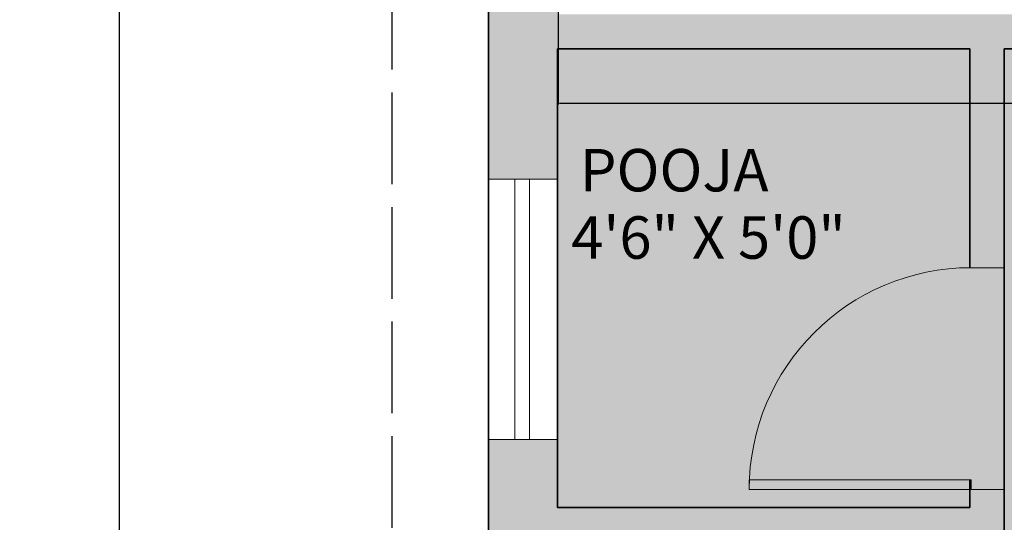
# Model space of a CAD drawing. Units: inches. Extents: x 1316 to 1777, y 813 to 1650.
# Tile 6 of 22: x 1316 to 1445, y 1368 to 1434. Entities that reach past the tile are written whole.
import ezdxf

# ---------------------------------------------------------------- set-up
doc = ezdxf.new("R2010")
doc.units = ezdxf.units.IN
doc.header["$MEASUREMENT"] = 0
doc.linetypes.add('ACAD_ISO02W100', pattern=[15, 12, -3])
for name, color, linetype, lineweight in [('A-ANNO-DIMS', 2, 'Continuous', 18), ('A-AREA-IDEN', 7, 'Continuous', 18), ('A-DOOR', 4, 'Continuous', 18), ('A-DOOR-PATT', 253, 'Continuous', 13), ('A-WALL-PATT', 250, 'Continuous', 13), ('C-PROP', 8, 'ACAD_ISO02W100', 25), ('walls', 250, 'Continuous', 35), ('windows', 141, 'Continuous', 18)]:
    doc.layers.add(name, color=color, linetype=linetype, lineweight=lineweight)
doc.layers.add('A-FLOR-PATT', color=254, linetype='Continuous', lineweight=13, true_color=0xfeeab9)
doc.styles.get("Standard").update_dxf_attribs({"font": 'arial.ttf'})
doc.dimstyles.get("Standard").update_dxf_attribs({"dimtxt": 7, "dimasz": 0.18, "dimexe": 0.18, "dimexo": 0.0625, "dimgap": 0.09, "dimtad": 0, "dimtih": 1, "dimtoh": 1, "dimzin": 0, "dimdsep": 46, "dimlunit": 3, "dimtxsty": 'Standard', "dimcen": 0.09, "dimadec": 0, "dimazin": 0, "dimtfac": 1, "dimtofl": 0, "dimtmove": 0, "dimatfit": 3, "dimfxl": 1, "dimtolj": 1, "dimtzin": 0, "dimarcsym": 0})

# ---------------------------------------------------------------- blocks, each defined once
blk = doc.blocks.new('*U15')
for p, q in [((0, 0), (-1e-16, -5.999999999999999)), ((40, -6e-16), (40, -6))]:
    blk.add_line(p, q)
blk.add_lwpolyline([(0, 0), (5.6e-15, 40), (1.750000000000007, 40), (1.749999999999998, -7e-16)], close=True)
blk.add_arc((0, 0), 40, 0, 90)
blk = doc.blocks.new('*D23')
at = {"layer": 'A-ANNO-DIMS', "color": 0, "lineweight": -2, "transparency": 16777216}
for p, q in [((1328.466746604303, 1604.172951843256), (1328.865516882555, 1604.172951843256)), ((1328.685516882555, 1603.992951843256), (1328.685516882555, 1282.594977494184)), ((1328.685516882555, 953.868981317008), (1328.685516882555, 1275.26695566608)), ((1328.466746604303, 953.688981317008), (1328.865516882556, 953.688981317008))]:
    blk.add_line(p, q, dxfattribs=at)
at = {"layer": 'A-ANNO-DIMS', "color": 0, "transparency": 16777216}
for points in [[(1328.655516882555, 1603.992951843256), (1328.715516882555, 1603.992951843256), (1328.685516882555, 1604.172951843256)], [(1328.655516882556, 953.868981317008), (1328.715516882555, 953.868981317008), (1328.685516882555, 953.688981317008)]]:
    blk.add_solid(points, dxfattribs=at)
at = {"layer": 'Defpoints', "color": 0, "transparency": 16777216}
for p in [(1328.404246604303, 1604.172951843256), (1328.404246604303, 953.688981317008), (1328.685516882555, 953.688981317008)]:
    blk.add_point(p, dxfattribs=at)
at = {"layer": 'A-ANNO-DIMS', "color": 0, "transparency": 16777216, "insert": (1328.685516882555, 1278.930966580132), "char_height": 7, "width": 24.3281036834925, "attachment_point": 5}
blk.add_mtext('\\A1;47\'-0"', dxfattribs=at)
blk = doc.blocks.new('*D30')
at = {"layer": 'A-ANNO-DIMS', "color": 0, "lineweight": -2, "transparency": 16777216}
for p, q in [((1386.153353095512, 1434.699095169867), (1386.153353095512, 1422.57802783725)), ((1466.177135312958, 1434.699095169867), (1466.177135312958, 1422.57802783725)), ((1386.333353095512, 1422.75802783725), (1465.997135312959, 1422.75802783725)), ((1466.177135312958, 1422.75802783725), (1466.357135312958, 1422.75802783725))]:
    blk.add_line(p, q, dxfattribs=at)
at = {"layer": 'A-ANNO-DIMS', "color": 0, "transparency": 16777216}
for points in [[(1386.333353095512, 1422.78802783725), (1386.333353095512, 1422.72802783725), (1386.153353095512, 1422.75802783725)], [(1465.997135312959, 1422.78802783725), (1465.997135312959, 1422.72802783725), (1466.177135312958, 1422.75802783725)]]:
    blk.add_solid(points, dxfattribs=at)
at = {"layer": 'Defpoints', "color": 0, "transparency": 16777216}
for p in [(1386.153353095512, 1434.761595169867), (1466.177135312958, 1434.761595169867), (1466.177135312958, 1422.75802783725)]:
    blk.add_point(p, dxfattribs=at)
at = {"layer": 'A-ANNO-DIMS', "color": 0, "transparency": 16777216, "insert": (1518.078103935059, 1422.75802783725), "char_height": 7, "attachment_point": 5}
blk.add_mtext('\\A1;WARDROBE 6\'-8" TYP.', dxfattribs=at)
blk = doc.blocks.new('*D36')
at = {"layer": 'A-ANNO-DIMS', "color": 0, "lineweight": -2, "transparency": 16777216}
for p, q in [((1416.108011424953, 1349.392697936214), (1416.108011424953, 1345.951925450247)), ((1438.2631613314, 1349.392697936214), (1438.2631613314, 1345.951925450247)), ((1416.288011424953, 1346.131925450247), (1438.0831613314, 1346.131925450247)), ((1438.2631613314, 1346.131925450247), (1438.443161331401, 1346.131925450247))]:
    blk.add_line(p, q, dxfattribs=at)
at = {"layer": 'A-ANNO-DIMS', "color": 0, "transparency": 16777216}
for points in [[(1416.288011424953, 1346.161925450247), (1416.288011424953, 1346.101925450247), (1416.108011424953, 1346.131925450247)], [(1438.0831613314, 1346.161925450247), (1438.0831613314, 1346.101925450247), (1438.2631613314, 1346.131925450247)]]:
    blk.add_solid(points, dxfattribs=at)
at = {"layer": 'Defpoints', "color": 0, "transparency": 16777216}
for p in [(1416.108011424953, 1349.455197936214), (1438.2631613314, 1349.455197936214), (1438.2631613314, 1346.131925450247)]:
    blk.add_point(p, dxfattribs=at)
at = {"layer": 'A-ANNO-DIMS', "color": 0, "transparency": 16777216, "insert": (1493.434934864825, 1346.131925450247), "char_height": 7, "attachment_point": 5}
blk.add_mtext('\\A1;WALL BASIN 1\'-10" TYP.', dxfattribs=at)

msp = doc.modelspace()

# ---------------------------------------------------------------- hatches: boundary and pattern name
at = {"layer": 'A-DOOR-PATT'}
h = msp.add_hatch(color=256, dxfattribs=at)
h.dxf.hatch_style = 1
h.paths.add_polyline_path([(1440.064450217018, 1373.459281729462), (1411.195884528974, 1373.459281729462, 0.0109414287710455), (1411.168078720428, 1372.18876759644), (1440.064450217018, 1372.18876759644)])
h.paths.add_polyline_path([(1505.845136951899, 1441.821674157348), (1476.976571263855, 1441.821674157348, 0.0109414287710455), (1476.948765455309, 1440.551160024325), (1505.845136951899, 1440.551160024325)])
h.paths.add_polyline_path([(1510.345136951899, 1469.591483064839), (1505.989088495822, 1469.591483064839, 0.0012392441961977), (1505.845136951899, 1469.59112628206), (1505.845136951899, 1441.821674157348), (1505.989088495822, 1441.821674157348), (1505.989088495822, 1440.551160024325), (1510.345136951899, 1440.551160024325)])
at = {"layer": 'A-FLOR-PATT'}
h = msp.add_hatch(color=256, dxfattribs=at)
h.dxf.hatch_style = 1
h.paths.add_polyline_path([(1567.673142217696, 1281.369300926962), (1651.673142217696, 1281.369300926962), (1651.673142217696, 1365.369300926962), (1597.673142217696, 1365.369300926962), (1597.673142217696, 1429.869300926962), (1570.345136951899, 1429.869300926962), (1570.345136951899, 1471.869300926962), (1510.345136951899, 1471.869300926962), (1510.345136951899, 1429.869300926962), (1444.564450217018, 1429.869300926962), (1444.564450217018, 1322.882360660317), (1444.564450217018, 1300.087519887597), (1510.564450217018, 1300.087519887597), (1510.564450217018, 1295.093869264817), (1510.564450217018, 1240.869300926962), (1386.064450217018, 1240.869300926962), (1386.064450217018, 1171.184826128129), (1400.961298831769, 1171.184826128129), (1400.961298831769, 1106.74181853581), (1386.064450217018, 1106.74181853581), (1386.064450217018, 1072.869300926962), (1510.564450217018, 1072.869300926962), (1510.564450217018, 1040.172951843256), (1541.068383692007, 1040.172951843256, -0.367085007058701), (1572.764174999282, 1069.546549507821), (1572.764174999282, 1069.578525976929), (1574.225256623933, 1069.578525976929), (1574.225256623933, 1040.172951843256), (1616.037285953149, 1040.172951843256), (1616.037285953149, 1086.627161740109), (1616.037285953149, 1103.704513499145), (1613.066060418845, 1105.234780569291), (1616.037285953149, 1106.685539866415), (1616.037285953149, 1123.869300926962), (1567.673142217696, 1123.869300926962)])
h.paths.add_polyline_path([(1508.987494855724, 1198.018101264616), (1511.117481528599, 1198.018101264616), (1511.117481528599, 1200.148087937491), (1532.594847146751, 1200.148087937491), (1532.594847146751, 1198.018101264616), (1534.724833819626, 1198.018101264616), (1534.724833819626, 1176.008238978245), (1530.464860473877, 1176.008238978245), (1530.464860473877, 1176.71823453587), (1513.247468201473, 1176.71823453587), (1513.247468201473, 1176.008238978245), (1508.987494855724, 1176.008238978245)], flags=16)
h.paths.add_polyline_path([(1505.978911344017, 1151.314990471522), (1521.503967005494, 1151.314990471522), (1521.503967005494, 1123.622553675171), (1505.978911344017, 1123.622553675171)], flags=16)
h.paths.add_polyline_path([(1507.734238645614, 1150.100746953806, -1), (1506.932299902515, 1150.100746953806, -1)], flags=0)
h.paths.add_polyline_path([(1512.288074001727, 1138.353334368216), (1512.279600715468, 1138.392440283947), (1512.219350358134, 1138.376242249414)], flags=0)
h.paths.add_polyline_path([(1511.538708600003, 1138.926307509397), (1511.801586230713, 1138.967144364025), (1511.816822451641, 1139.269704188439), (1511.606794574277, 1139.246286533845)], flags=0)
h.paths.add_polyline_path([(1513.744555260512, 1140.234298321423), (1513.680232363733, 1139.885116881769), (1514.013725426534, 1140.045442118172), (1513.85452204526, 1140.307851476896)], flags=0)
h.paths.add_polyline_path([(1513.759454991183, 1139.088508933479), (1514.004707571892, 1139.255238426424), (1513.806733823314, 1139.482778214552), (1513.564128907831, 1139.327271464974)], flags=0)
h.paths.add_polyline_path([(1514.219475210051, 1138.385213274156), (1514.335730050378, 1138.330012877603), (1514.544443105969, 1138.319719602207), (1514.802071501717, 1138.873746829037), (1514.451386945615, 1138.715560522777)], flags=0)
h.paths.add_polyline_path([(1514.576784523415, 1137.439218133731), (1514.572807725035, 1137.400121795131), (1514.699202201671, 1137.400121795131), (1514.696265725507, 1137.401958254237)], flags=0)
h.paths.add_polyline_path([(1512.259630054145, 1136.199252443718), (1512.198645006043, 1136.399020086717), (1512.031969302785, 1136.324884611944), (1512.095408670439, 1136.101205019573), (1512.257489338984, 1136.192116726515)], flags=0)
h.paths.add_polyline_path([(1512.643663084783, 1137.273739653883), (1512.355504649132, 1137.230281342332), (1512.431954114942, 1137.048783229095), (1512.702875297586, 1137.092989450977)], flags=0)
h.paths.add_polyline_path([(1513.048588650928, 1137.592520798729), (1512.979298324136, 1137.799799709794), (1512.842806872769, 1137.757466697763), (1512.887278702865, 1137.556025839099)], flags=0)
h.paths.add_polyline_path([(1513.269281623239, 1138.555876366321), (1513.570749546786, 1137.962332598873), (1513.458764523686, 1136.814048268166), (1513.212081965274, 1137.877990637943), (1513.032322366809, 1138.442602014432)], flags=0)
h.paths.add_polyline_path([(1514.891020715756, 1136.377090047208), (1514.695899864911, 1136.400535518201), (1514.682939550409, 1136.245500587688), (1514.870369662043, 1136.165423867704)], flags=0)
h.paths.add_polyline_path([(1514.142311807212, 1137.292647657223), (1514.047049214511, 1136.74320071616), (1514.270411313405, 1136.750949401328), (1514.327746372416, 1137.265481105849)], flags=0)
h.paths.add_polyline_path([(1515.361925908058, 1138.975942407129), (1515.333738674027, 1138.638448296537), (1515.595602136156, 1138.588081597507), (1515.627104749056, 1138.931608018565)], flags=0)
h.paths.add_polyline_path([(1537.284795120854, 1177.912388692567), (1537.994790678479, 1177.912388692567), (1537.994790678479, 1195.129780964971), (1537.284795120854, 1195.129780964971), (1537.284795120854, 1199.38975431072), (1559.294657407225, 1199.38975431072), (1559.294657407225, 1197.259767637845), (1561.4246440801, 1197.259767637845), (1561.4246440801, 1175.782402019693), (1559.294657407225, 1175.782402019693), (1559.294657407225, 1173.652415346818), (1559.378615070445, 1173.652415346818), (1559.378615070445, 1171.514303738793), (1561.51672667847, 1171.514303738793), (1561.51672667847, 1098.818509065945), (1559.378615070445, 1098.818509065945), (1559.378615070445, 1096.68039745792), (1537.284795120854, 1096.68039745792), (1537.284795120854, 1100.95662067397), (1537.997498990196, 1100.95662067397), (1537.997498990196, 1169.376192130768), (1537.284795120854, 1169.376192130768), (1537.284795120854, 1173.652415346818)], flags=16)
h.paths.add_polyline_path([(1518.623279367581, 1345.565265318288), (1519.133216999197, 1345.479657117201), (1519.133247129367, 1345.484585273925), (1518.623292796693, 1345.567461813277)], flags=16)
h.paths.add_polyline_path([(1518.798043157878, 1374.150014517315), (1519.307980789494, 1374.064406316228), (1519.308010919664, 1374.069334472953), (1518.79805658699, 1374.152211012305)], flags=16)
h.paths.add_polyline_path([(1537.763945546351, 1413.501272593833), (1537.678419015976, 1412.991334462891), (1537.683273643974, 1412.991304782267), (1537.76615767817, 1413.501259069119)], flags=16)
h.paths.add_polyline_path([(1572.904903294898, 1373.821409718101), (1573.926762419731, 1373.974678074354), (1574.026627442758, 1390.308820473798), (1573.007147246318, 1390.474521481455), (1573.006718884663, 1390.474591095266)], flags=16)
h.paths.add_polyline_path([(1572.730139504601, 1345.236660519073), (1573.751998629434, 1345.389928875326), (1573.851863652461, 1361.72407127477), (1572.832383456021, 1361.889772282427), (1572.831955094366, 1361.889841896238)], flags=16)
h.paths.add_polyline_path([(1537.210658487583, 1322.64259197221), (1537.363943428096, 1321.620732745983), (1553.69808582754, 1321.520867722956), (1553.863838585734, 1322.540776390265)], flags=16)
h.paths.add_polyline_path([(1535.907853535946, 1331.328394679552), (1527.214399285865, 1331.381545435045), (1527.663791889487, 1404.885186232545), (1564.415612288236, 1404.660489930734), (1563.966219684615, 1331.156849133235), (1555.272745017813, 1331.210000013553), (1553.946716560728, 1323.050730714162), (1537.134020158137, 1323.153521560007)], flags=16)
h.paths.add_polyline_path([(1536.149948378398, 1336.502989385165), (1536.235164066325, 1337.571577967879), (1536.323287084786, 1338.628101895201), (1536.410786509507, 1339.662781903015), (1536.494625364907, 1340.6698173033), (1536.573878305868, 1341.65983134291), (1536.648126641431, 1342.647834135966), (1536.716972722469, 1343.648937760143), (1536.780017027388, 1344.677948027938), (1536.836830656389, 1345.749875115879), (1536.91349345135, 1347.47536960008), (1536.930181129876, 1348.082213381731), (1536.86671979596, 1346.313806322279), (1536.754065794645, 1344.188314997416), (1536.618602559507, 1342.21851898877), (1536.494625364906, 1340.669817303289), (1536.410786509508, 1339.662781903024), (1536.323287084785, 1338.628101895196), (1536.235164066325, 1337.571577967878), (1536.149948378398, 1336.502989385167), (1536.071202820108, 1335.432319400725), (1536.002480605875, 1334.369653419014), (1535.917201218224, 1332.754159960459), (1535.909282823342, 1332.307756473361), (1535.96435308899, 1333.780079645636), (1536.071202820108, 1335.432319400726)], flags=0)
h.paths.add_polyline_path([(1540.411728678358, 1338.345220732376), (1540.538507986221, 1339.036732867615), (1540.667450686668, 1339.758144792479), (1540.798139602249, 1340.51803480286), (1540.930104638842, 1341.324675241543), (1541.06290820131, 1342.186644529235), (1541.195663950278, 1343.109256879628), (1541.325751198274, 1344.084667215432), (1541.450112594895, 1345.102072455087), (1541.565699126105, 1346.150363189455), (1541.669432399664, 1347.218634373414), (1541.758274858692, 1348.295980712192), (1541.829158319786, 1349.371497098253), (1541.87902418423, 1350.434176273261), (1541.905658245644, 1351.475864398132), (1541.910264078201, 1352.499718972741), (1541.894848813054, 1353.511751165878), (1541.861450207875, 1354.517971959091), (1541.812104772023, 1355.524188157142), (1541.748831093802, 1356.536615043187), (1541.673675267255, 1357.560957271187), (1541.551221046702, 1359.062282646612), (1541.495486505545, 1359.670454934914), (1541.588655256529, 1358.603328035907), (1541.721318618915, 1356.976835527602), (1541.846114060333, 1354.980013725856), (1541.912433480836, 1352.981966815021), (1541.903299375855, 1350.951498912638), (1541.805645357175, 1348.870418133965), (1541.627733180341, 1346.712969607265), (1541.39605931794, 1344.611846225434), (1541.135168242209, 1342.655652549989), (1540.871929016276, 1340.947082961546), (1540.617179283622, 1339.465841984599), (1540.411728678363, 1338.345220732389), (1540.287580984743, 1337.67502977883), (1540.166494164132, 1337.01788791383), (1540.048925605183, 1336.365114503449), (1539.936674201221, 1335.710368832696), (1539.836864251217, 1335.055036635329), (1539.758020939376, 1334.402536924379), (1539.708629238703, 1333.756391050932), (1539.697173498044, 1333.120018277682), (1539.75093556766, 1332.162191347439), (1539.822087714565, 1331.89006440645), (1539.690956844971, 1332.774679737417), (1539.713650637448, 1334.035332547662), (1539.86680860596, 1335.30285325234), (1540.085210789094, 1336.576760560778), (1540.287580984743, 1337.67502977883)], flags=0)
h.paths.add_polyline_path([(1545.598581542273, 1331.583674047033), (1545.601408931398, 1331.616855477121), (1545.614142276281, 1331.689058908809), (1545.736718477884, 1332.197227143153), (1545.766951209007, 1332.331509735297), (1545.840044120643, 1332.681341212682), (1545.924609388668, 1333.114205605127), (1546.015565858785, 1333.613901317454), (1546.107830504227, 1334.163920489319), (1546.196310713542, 1334.747857411176), (1546.27592408412, 1335.349306311069), (1546.341588213349, 1335.951861417042), (1546.388220074462, 1336.539014868746), (1546.411904372759, 1337.098233262493), (1546.413511757999, 1337.631655211558), (1546.395048737181, 1338.145189796344), (1546.358553067975, 1338.644847998394), (1546.30606313221, 1339.136742887642), (1546.239595021565, 1339.626681393686), (1546.161196702551, 1340.120674435653), (1546.072884891005, 1340.624631031533), (1545.887738197254, 1341.63015699768), (1545.717659533451, 1342.62070013092), (1545.546853733249, 1343.94500888803), (1545.431881256549, 1345.533720124316), (1545.403899849759, 1347.401905451854), (1545.417510423816, 1348.013069267128), (1545.410556413592, 1346.957478372932), (1545.425070640934, 1345.988432507364), (1545.462877367243, 1345.105410056077), (1545.521092971858, 1344.300975918152), (1545.595702123642, 1343.566272620922), (1545.68263719895, 1342.892238827028), (1545.777872657803, 1342.270017126221), (1545.877351709551, 1341.690648207114), (1545.977037981224, 1341.145172633476), (1546.133225269608, 1340.296924301995), (1546.32712189736, 1339.07516870602), (1546.43378476773, 1337.614859053002), (1546.377188266119, 1336.278538916938), (1546.246417261819, 1335.078542247844), (1546.032296532176, 1333.665423983985), (1545.840044120643, 1332.681341212682), (1545.766951209007, 1332.331509735297)], flags=0)
h.paths.add_polyline_path([(1551.802739251137, 1337.655775652498), (1551.96257269545, 1338.249893918501), (1552.102195298518, 1338.801154932478), (1552.224958021371, 1339.338328209144), (1552.330696453755, 1339.864579612065), (1552.418402861907, 1340.377056720641), (1552.487067639598, 1340.872600849098), (1552.535672844225, 1341.34835963925), (1552.563199284875, 1341.801276556129), (1552.568639227787, 1342.228499179132), (1552.550972857889, 1342.626868884903), (1552.509678498417, 1342.994551203202), (1552.446288501197, 1343.33337442512), (1552.362792521005, 1343.646491244529), (1552.261208966661, 1343.936747902882), (1552.143557495304, 1344.207194818415), (1552.011836098078, 1344.460678357413), (1551.868075265113, 1344.700350964085), (1551.746105860759, 1344.881722683215), (1550.887297650741, 1346.05192221882), (1550.42788872704, 1347.125680184261), (1550.183287427721, 1348.353333686171), (1550.047936052465, 1349.632359022536), (1549.978096005541, 1351.223542107026), (1549.974102148838, 1353.140827975589), (1549.989226669163, 1353.748427546368), (1549.975058438592, 1352.681752708607), (1549.977087298692, 1351.70778065901), (1549.995607655661, 1350.824569845699), (1550.030618304039, 1350.026913573531), (1550.082058657804, 1349.309911787039), (1550.149928759809, 1348.668561967865), (1550.234168024029, 1348.097964060535), (1550.334775869163, 1347.593013458303), (1550.451691709185, 1347.148810105696), (1550.584412233058, 1346.759844100773), (1550.73038050297, 1346.418678345312), (1550.88655602074, 1346.117266144286), (1551.049909745336, 1345.847764917032), (1551.217401178577, 1345.602127968521), (1551.385990446439, 1345.372410692116), (1551.55262809021, 1345.150770631988), (1552.000038284146, 1344.537104232464), (1552.453505275841, 1343.494713960715), (1552.591463897673, 1342.266339273388), (1552.508711326437, 1340.904737898757), (1552.245597777252, 1339.367339734202), (1551.924893638995, 1338.101128644033), (1551.618511514029, 1336.984114361546), (1551.405674157756, 1336.200020283199), (1551.009764092749, 1334.698598399404), (1550.877399289293, 1334.154667887629), (1551.263664389663, 1335.676855458292), (1551.618511514027, 1336.984114361536)], flags=0)
h.paths.add_polyline_path([(1558.642358998526, 1348.348341932098), (1558.795153425402, 1348.811416841303), (1558.918173552255, 1349.215358215379), (1559.008026171039, 1349.574581801048), (1559.061298904339, 1349.903707646641), (1559.075825921932, 1350.214183320864), (1559.054343192669, 1350.505992096326), (1559.00083323259, 1350.775944766007), (1558.919250427844, 1351.021260663692), (1558.81356708563, 1351.238750644777), (1558.687756761463, 1351.425429741436), (1558.545793010855, 1351.578312985846), (1558.391628971643, 1351.694415535011), (1558.228764001313, 1351.771674150153), (1558.05869086465, 1351.812121548804), (1557.882428128411, 1351.81871217754), (1557.700994359352, 1351.79440048294), (1557.515397915392, 1351.742140973996), (1557.326668820441, 1351.665092211649), (1557.135793766425, 1351.566004652943), (1556.943823194933, 1351.44803673399), (1556.751584825563, 1351.314654529213), (1556.741969848742, 1351.307485185875), (1556.174649390243, 1350.878470713214), (1555.982386678774, 1350.741107061228), (1555.790208852573, 1350.61762743028), (1555.103431920574, 1350.247624890473), (1554.019478994433, 1350.696346369238), (1553.658410413117, 1351.73359972735), (1553.592207666961, 1352.861368347784), (1553.704659497418, 1354.248209262139), (1553.753119918252, 1354.656598557367), (1553.684819216316, 1354.00352392911), (1553.637913725648, 1353.425049987856), (1553.614699631385, 1352.917691559993), (1553.614827379228, 1352.476039895736), (1553.637249468889, 1352.094077959223), (1553.680938817757, 1351.765788589762), (1553.744858758541, 1351.485256777466), (1553.82798220863, 1351.246465361642), (1553.929261667735, 1351.043397306428), (1554.04767130156, 1350.870239627912), (1554.182026927633, 1350.721997047951), (1554.330490954936, 1350.598680801359), (1554.491077653114, 1350.501119766308), (1554.661792955443, 1350.430449148551), (1554.840661964566, 1350.387599852234), (1555.02568040492, 1350.373707145527), (1555.214873379145, 1350.389701932573), (1555.406255781046, 1350.436515179933), (1555.598153361026, 1350.514157123772), (1555.790208852573, 1350.61762743028), (1555.982386678773, 1350.741107061227), (1556.174649390244, 1350.878470713214), (1556.366961410069, 1351.02389934801), (1556.559285288865, 1351.171267662216), (1556.751584825563, 1351.314654529213), (1556.943823194933, 1351.44803673399), (1557.135793766425, 1351.566004652943), (1557.326668820441, 1351.665092211648), (1558.042515074605, 1351.95733685961), (1558.893728230531, 1351.316279335487), (1559.136865914879, 1350.089672795452), (1558.886015641058, 1349.086793457618), (1558.642358998525, 1348.348341932093), (1558.463193064356, 1347.811615590227), (1558.261048830942, 1347.186822068983), (1558.03933929985, 1346.459443408408), (1557.677450203418, 1345.174834336041), (1557.548968991007, 1344.635807724703), (1557.908545731516, 1346.030339390738), (1558.328508124364, 1347.408140702653)], flags=0)
h.paths.add_polyline_path([(1562.145123345359, 1353.919129120074), (1562.250304117219, 1354.679787637482), (1562.34093833006, 1355.343853771733), (1562.416101040585, 1355.923686334763), (1562.475035862508, 1356.430826370303), (1562.517611688201, 1356.872216949942), (1562.54387555173, 1357.25388122627), (1562.553854069482, 1357.581842476714), (1562.547593651368, 1357.862021765479), (1562.525120913776, 1358.10044236999), (1562.486482890773, 1358.30312744284), (1562.431704950433, 1358.475896084676), (1562.361155192264, 1358.623850655281), (1562.276503898586, 1358.748001864806), (1562.179752001843, 1358.848337479786), (1562.072869183806, 1358.924743365611), (1561.957877418753, 1358.977309252376), (1561.836746388454, 1359.005921005473), (1561.71148785835, 1359.010668417409), (1561.584092552045, 1358.991539317136), (1561.456045120288, 1358.949239273116), (1561.341584300566, 1358.895014406292), (1560.779829007024, 1358.553784684453), (1560.630616275888, 1358.472819004295), (1560.474487483611, 1358.402819474164), (1560.311154867376, 1358.348484094885), (1559.637466910391, 1358.206630908504), (1558.973121038646, 1358.903907683205), (1558.815552073528, 1360.002456271339), (1558.803942930122, 1361.236291863163), (1558.829841213422, 1361.673699707903), (1558.80694301689, 1360.917438550413), (1558.812784665874, 1360.296580130481), (1558.845278068372, 1359.795210830316), (1558.902335132382, 1359.397417032129), (1558.981856932905, 1359.087183092155), (1559.081756002095, 1358.848697480995), (1559.199942999639, 1358.66584240408), (1559.334180223548, 1358.524951186848), (1559.481597784608, 1358.420834672959), (1559.639186392453, 1358.350550586885), (1559.803946965561, 1358.311156590683), (1559.97287021357, 1358.299710408824), (1560.142945597805, 1358.313065589002), (1560.311154867377, 1358.348484094885), (1560.474487483611, 1358.402819474164), (1560.630616275888, 1358.472819004295), (1560.779829007024, 1358.553784684454), (1560.923096183733, 1358.640810155187), (1561.061387688574, 1358.728886968651), (1561.195663195268, 1358.813006739421), (1561.382100208996, 1358.919625179564), (1561.341584300566, 1358.895014406292), (1561.972476451099, 1359.193894345525), (1562.53631106285, 1358.366963698877), (1562.559911530188, 1357.31074636116), (1562.455247211757, 1356.225674176933), (1562.323097858171, 1355.206225864646), (1562.145123345359, 1353.91912912008), (1562.026320333625, 1353.049417319218), (1561.815039989057, 1351.456922136686), (1561.751502783429, 1350.932786338753), (1561.948339842468, 1352.478551712307)], flags=0)
h.paths.add_polyline_path([(1572.764174999282, 1069.546549507821, 0.3670850070587006), (1541.068383692007, 1040.172951843256), (1572.764174999282, 1040.172951843256)], flags=17)
h.paths.add_polyline_path([(1572.764174999282, 1040.172951843256), (1541.068383692007, 1040.172951843256, 0.0299535364659094), (1540.829105203347, 1036.182374556343), (1540.829105203347, 1031.172951843255), (1574.225256623933, 1031.172951843255), (1574.225256623933, 1036.182374556343), (1572.764174999282, 1036.182374556343)])
h = msp.add_hatch(color=256, dxfattribs=at)
h.dxf.hatch_style = 1
h.paths.add_polyline_path([(1440.064450217018, 1429.869300926962), (1386.064450217018, 1429.869300926962), (1386.064450217018, 1369.869300926962), (1440.064450217018, 1369.869300926962), (1440.064450217018, 1372.18876759644), (1411.168078720428, 1372.18876759644), (1411.168078720428, 1373.459281729462), (1411.195884528974, 1373.459281729462, -0.4000144639257879), (1440.064450217018, 1401.228733854174)])
h.paths.add_polyline_path([(1444.564450217018, 1401.229090636953), (1440.208401760941, 1401.229090636953, 0.4014527144963568), (1411.195884528974, 1373.459281729462), (1440.208401760941, 1373.459281729462), (1440.208401760941, 1372.18876759644), (1444.564450217018, 1372.18876759644)])
at = {"layer": 'A-WALL-PATT'}
h = msp.add_hatch(color=256, dxfattribs=at)
h.dxf.hatch_style = 1
h.paths.add_polyline_path([(1713.173142217696, 1281.369300926962), (1656.173142217696, 1281.369300926962), (1656.173142217696, 1298.257717658217), (1651.673142217696, 1298.257717658217), (1651.673142217696, 1281.369300926962), (1567.673142217696, 1281.369300926962), (1567.673142217696, 1266.995117174766), (1572.173142217695, 1266.995117174766), (1572.173142217695, 1276.869300926963), (1704.173142217696, 1276.869300926962), (1704.173142217696, 1132.869300926962), (1608.640148269009, 1132.869300926962), (1608.640148269009, 1123.869300926962), (1704.173142217696, 1123.869300926962), (1704.173142217696, 1040.172951843256), (1652.868762127258, 1040.172951843256), (1652.868762127258, 1031.172951843254), (1713.173142217696, 1031.172951843253), (1713.173142217696, 1040.172951843256)])
h.paths.add_polyline_path([(1572.173142217696, 1237.954794134253), (1567.673142217696, 1237.954794134253), (1567.673142217696, 1123.869300926962), (1583.145592691861, 1123.869300926962), (1583.145592691861, 1132.869300926963), (1572.173142217696, 1132.869300926963)], flags=17)
h.paths.add_polyline_path([(1510.345136951899, 1566.369300926962), (1524.170902149835, 1566.369300926962), (1524.170902149835, 1571.984613741441), (1524.170902149835, 1575.369300926961), (1445.954793584458, 1575.369300926961), (1445.954793584458, 1566.369300926962), (1505.845136951899, 1566.369300926962), (1505.845136951899, 1469.591483064839), (1510.345136951899, 1469.591483064839), (1510.345136951899, 1471.869300926962), (1529.081211183796, 1471.869300926962), (1529.081211183796, 1476.369300926962), (1510.345136951899, 1476.369300926962)])
h.paths.add_polyline_path([(1609.722471703215, 1575.369300926961), (1545.118796217357, 1575.369300926961), (1545.118796217357, 1566.369300926962), (1570.345136951899, 1566.369300926962), (1570.345136951899, 1476.369300926962), (1562.477362604382, 1476.369300926962), (1562.477362604382, 1471.869300926962), (1570.345136951899, 1471.869300926962), (1570.345136951899, 1469.591483064839), (1574.845136951899, 1469.591483064839), (1574.845136951899, 1566.369300926962), (1609.722471703215, 1566.369300926962)])
h.paths.add_polyline_path([(1713.173142217696, 1575.369300926961), (1655.232651300773, 1575.369300926961), (1655.232651300773, 1566.369300926962), (1704.173142217696, 1566.369300926962), (1704.173142217696, 1434.369300926962), (1574.845136951899, 1434.369300926962), (1574.845136951899, 1440.551160024325), (1574.701185407976, 1440.551160024325), (1570.345136951899, 1440.551160024325), (1570.345136951899, 1429.869300926962), (1597.673142217696, 1429.869300926962), (1597.673142217696, 1408.281186528541), (1602.173142217695, 1408.281186528541), (1602.173142217695, 1429.869300926962), (1704.173142217696, 1429.869300926962), (1704.173142217696, 1410.703982852585), (1707.374745037781, 1410.703982852585), (1713.173142217696, 1410.703982852585)])
h.paths.add_polyline_path([(1713.173142217696, 1383.675544097327), (1704.173142217696, 1383.675544097327), (1704.173142217696, 1369.869300926962), (1602.173142217696, 1369.869300926962), (1602.173142217695, 1379.240863488028), (1597.673142217696, 1379.240863488028), (1597.673142217696, 1365.369300926962), (1713.173142217696, 1365.369300926962)])
h.paths.add_polyline_path([(1444.564450217018, 1429.869300926962), (1510.345136951899, 1429.869300926962), (1510.345136951899, 1440.551160024325), (1505.845136951899, 1440.551160024325), (1505.845136951899, 1434.369300926962), (1386.064450217018, 1434.369300926961), (1386.064450217018, 1566.369300926962), (1400.4446139869, 1566.369300926962), (1400.4446139869, 1575.369300926961), (1377.064450217018, 1575.369300926961), (1377.064450217018, 1412.813262305812), (1380.508552477466, 1412.813262305812), (1386.064450217018, 1412.813262305812), (1386.064450217018, 1429.869300926962), (1440.064450217018, 1429.869300926962), (1440.064450217018, 1401.229090636953), (1444.564450217018, 1401.229090636953)])
h.paths.add_polyline_path([(1444.564450217018, 1372.18876759644), (1440.064450217018, 1372.18876759644), (1440.064450217018, 1369.869300926962), (1386.064450217018, 1369.869300926962), (1386.064450217018, 1378.757622609401), (1377.064450217018, 1378.757622609401), (1377.064450217018, 1349.201183977028), (1381.117947355797, 1349.201183977028), (1386.064450217018, 1349.201183977028), (1386.064450217018, 1365.369300926962), (1440.064450217018, 1365.369300926962), (1440.064450217018, 1322.882360660317), (1444.564450217018, 1322.882360660317)])
h.paths.add_polyline_path([(1510.564450217018, 1295.093869264817), (1506.064450217018, 1295.093869264817), (1506.064450217018, 1245.369300926962), (1386.064450217018, 1245.369300926962), (1386.064450217018, 1272.58216425724), (1377.064450217018, 1272.58216425724), (1377.064450217018, 1212.904590025772), (1380.100240558029, 1212.904590025772), (1386.064450217018, 1212.904590025772), (1386.064450217018, 1240.869300926962), (1510.564450217018, 1240.869300926962)])
h.paths.add_polyline_path([(1386.064450217018, 1163.761289951094), (1377.064450217018, 1163.761289951094), (1377.064450217018, 1063.869300926961), (1419.36334498438, 1063.869300926961), (1419.36334498438, 1072.869300926962), (1386.064450217018, 1072.869300926962)])
h.paths.add_polyline_path([(1510.564450217018, 1072.869300926962), (1469.381492401113, 1072.869300926962), (1469.381492401113, 1063.869300926961), (1501.564450217018, 1063.869300926962), (1501.564450217018, 1033.022564166395), (1501.564450217018, 1031.172951843256), (1540.829105203347, 1031.172951843255), (1540.829105203347, 1036.182374556343, -0.0299535364659092), (1541.068383692007, 1040.172951843256), (1510.564450217018, 1040.172951843256)])
h.paths.add_polyline_path([(1607.368796217357, 1040.172951843256), (1574.225256623933, 1040.172951843256), (1574.225256623933, 1036.182374556343), (1574.225256623933, 1031.172951843255), (1607.368796217357, 1031.172951843254)], flags=17)
h.paths.add_polyline_path([(1637.054389108292, 1040.172951843256), (1624.70577568894, 1040.172951843256), (1624.70577568894, 1031.172951843254), (1637.054389108293, 1031.172951843254)], flags=17)

# ---------------------------------------------------------------- linework, layer by layer
at = {"layer": 'C-PROP'}
msp.add_line((1364.398563382318, 1604.172951843256), (1364.398563382318, 953.6889813170072), dxfattribs=at)
at = {"layer": 'walls'}
for p, q in [((1377.064450217018, 1575.369300926961), (1377.064450217018, 953.6889813170072)), ((1386.064450217018, 1429.869300926962), (1440.064450217018, 1429.869300926962)), ((1386.064450217018, 1429.869300926962), (1386.064450217018, 1369.869300926962)), ((1440.064450217018, 1429.869300926962), (1440.064450217018, 1401.228733854174)), ((1444.564450217018, 1429.869300926962), (1444.564450217018, 1322.882360660317)), ((1444.564450217018, 1429.869300926962), (1510.345136951899, 1429.869300926962)), ((1440.064450217018, 1373.459281729462), (1440.064450217018, 1369.869300926962)), ((1386.064450217018, 1369.869300926962), (1440.064450217018, 1369.869300926962))]:
    msp.add_line(p, q, dxfattribs=at)
at = {"layer": 'windows'}
for p, q in [((1377.064450217018, 1412.813262305812), (1386.064450217018, 1412.813262305812)), ((1377.064450217018, 1378.757622609401), (1377.064450217018, 1412.813262305812)), ((1377.064450217018, 1412.813262305812), (1380.508552477466, 1412.813262305812)), ((1380.508552477466, 1412.813262305812), (1380.508552477466, 1378.757622609401)), ((1382.399723177026, 1378.757622609401), (1382.399723177026, 1412.813262305812)), ((1386.064450217018, 1412.813262305812), (1386.064450217018, 1378.757622609401)), ((1386.064450217018, 1378.757622609401), (1377.064450217018, 1378.757622609401)), ((1380.508552477466, 1378.757622609401), (1382.399723177026, 1378.757622609401))]:
    msp.add_line(p, q, dxfattribs=at)

# ---------------------------------------------------------------- block references
at = {"layer": 'A-DOOR', "xscale": 0.7260080760128325, "yscale": 0.7260080760128325, "zscale": 0.7260080760128325, "rotation": 90}
msp.add_blockref('*U15', (1440.208401760941, 1372.18876759644), dxfattribs=at)

# ---------------------------------------------------------------- texts
at = {"layer": 'A-AREA-IDEN'}
for s, p in [('POOJA', (1389.010802448164, 1411.214113332788)), ('4\'6" X 5\'0"', (1387.87539217676, 1402.403546064756))]:
    msp.add_text(s, height=5.551774925409831, dxfattribs=at).set_placement(p)

# ---------------------------------------------------------------- dimensions: what is measured, and where the dimension line sits
at = {"layer": 'A-ANNO-DIMS'}
dim = msp.add_linear_dim(base=(1328.685516882555, 953.688981317008), p1=(1328.404246604303, 1604.172951843256), p2=(1328.404246604303, 953.6889813170077), angle=90, text='47\'-0"', dimstyle='Standard', override={"dimclrd": 0, "dimclre": 0, "dimclrt": 0}, dxfattribs=at)
dim.commit()
dim.dimension.update_dxf_attribs({"geometry": '*D23', "text_midpoint": (1328.685516882555, 1278.930966580132)})
for base, p1, p2, text, picture, middle in [((1466.177135312958, 1422.75802783725), (1386.153353095512, 1434.761595169867), (1466.177135312958, 1434.761595169867), 'WARDROBE <> TYP.', '*D30', (1518.078103935059, 1422.75802783725)), ((1438.2631613314, 1346.131925450247), (1416.108011424953, 1349.455197936214), (1438.2631613314, 1349.455197936214), 'WALL BASIN <> TYP.', '*D36', (1493.434934864825, 1346.131925450247))]:
    dim = msp.add_linear_dim(base=base, p1=p1, p2=p2, text=text, dimstyle='Standard', override={"dimdec": 1, "dimlfac": 1, "dimrnd": 0, "dimzin": 1, "dimdsep": 46, "dimlunit": 4, "dimfrac": 2}, dxfattribs=at)
    dim.commit()
    dim.dimension.update_dxf_attribs({"geometry": picture, "text_midpoint": middle})

doc.saveas('drawing.dxf')
